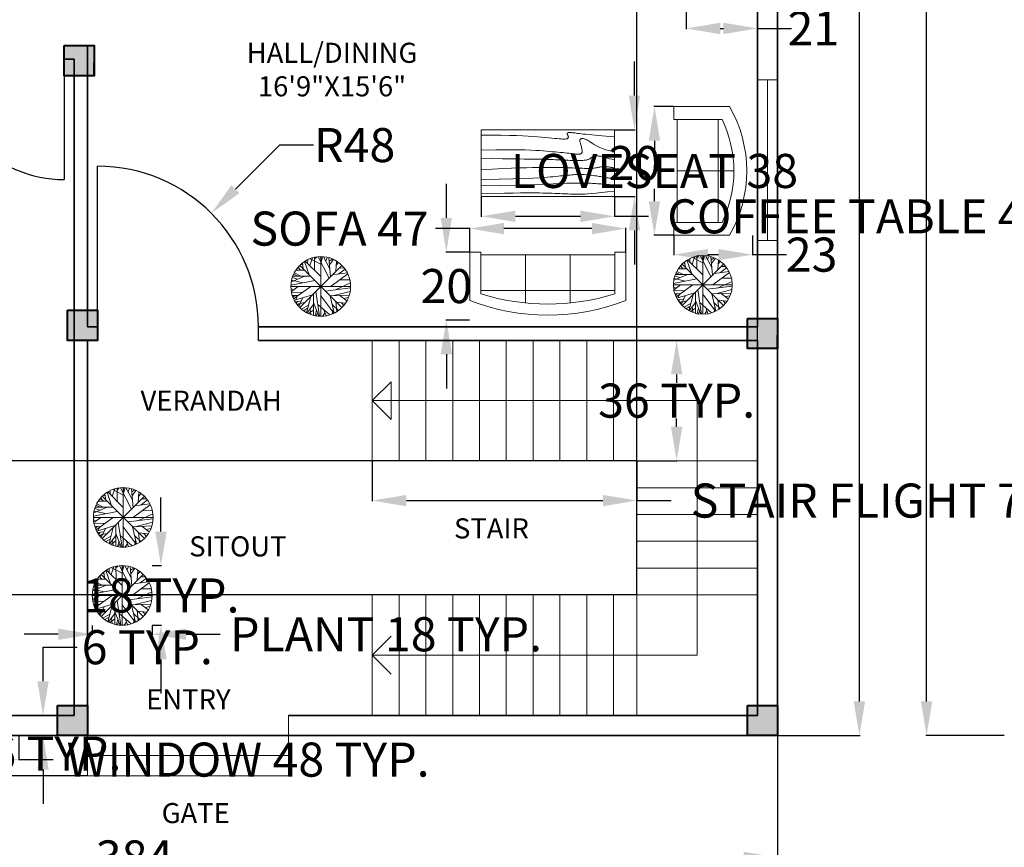
# Model space of a CAD drawing. Units: inches. Extents: x -107 to 647, y -210 to 500.
# Tile 4 of 7: x 183 to 477, y -31 to 216. Entities that reach past the tile are written whole.
import ezdxf

# ---------------------------------------------------------------- set-up
doc = ezdxf.new("R2010")
doc.units = ezdxf.units.IN
doc.header["$MEASUREMENT"] = 0
for name, color, linetype, lineweight in [('A-ANNO-DIMS', 2, 'Continuous', 18), ('A-ANNO-SYMB', 2, 'Continuous', 13), ('A-ANNO-TEXT', 7, 'Continuous', 18), ('A-AREA-IDEN', 7, 'Continuous', 18), ('A-COLS', 7, 'Continuous', 40), ('A-DOOR', 3, 'Continuous', 25), ('A-FLOR-STRS', 7, 'Continuous', 18), ('A-FURN', 8, 'Continuous', 18), ('A-GLAZ', 4, 'Continuous', 18), ('A-WALL', 7, 'Continuous', 35), ('L-PLNT', 3, 'Continuous', 13)]:
    doc.layers.add(name, color=color, linetype=linetype, lineweight=lineweight)
doc.styles.get("Standard").update_dxf_attribs({"font": 'arial.ttf'})
doc.dimstyles.get("Standard").update_dxf_attribs({"dimtxt": 10.18, "dimasz": 10.18, "dimexe": 0.18, "dimexo": 0.0625, "dimgap": 0.09, "dimtad": 0, "dimtih": 1, "dimtoh": 1, "dimdec": 0, "dimzin": 0, "dimdsep": 46, "dimlunit": 3, "dimtxsty": 'Standard', "dimcen": 0.09, "dimadec": 0, "dimazin": 0, "dimtfac": 1, "dimtdec": 0, "dimtofl": 0, "dimtmove": 0, "dimatfit": 3, "dimfxl": 1, "dimtolj": 1, "dimtzin": 0, "dimarcsym": 0})

# ---------------------------------------------------------------- blocks, each defined once
blk = doc.blocks.new('Sofa - Roundback 7 ft.')
for p, q in [((-12.00002, -32.4421), (-12.00003, -6.5971)), ((11.99997, -32.4421), (11.99998, -6.5971)), ((-36.000027, -34), (-36.000027, -11.4696)), ((-35.999844, -13.3819), (35.9998, -13.3819)), ((35.99998, -34), (35.99998, -11.4696)), ((-36.000027, -32.4421), (35.99998, -32.4421))]:
    blk.add_line(p, q)
for points in [[(-36.000027, -34), (-42.000027, -34), (-42.000027, -8)], [(41.99998, -8), (41.99998, -34), (35.99998, -34)]]:
    blk.add_lwpolyline(points)
for centre, radius, start, end in [((0, -114.25), 114.25, 68.43141, 111.5686), ((-0.00001, -127.1968), 121.1968, 72.72033, 107.2797)]:
    blk.add_arc(centre, radius, start, end)
blk = doc.blocks.new('Sofa - Roundback Loveseat 5 ft.')
for p, q in [((0, -32.44198), (0, -5.99998)), ((-24, -33.99998), (-24, -11.46958)), ((-23.9998, -13.38178), (23.99986, -13.38178)), ((24.00004, -33.99998), (24.00004, -11.46958)), ((-24, -32.44198), (24.00004, -32.44198))]:
    blk.add_line(p, q)
for points in [[(-24, -33.99998), (-30, -33.99998), (-30, -7.99998)], [(30.00004, -7.99998), (30.00004, -33.99998), (24.00004, -33.99998)]]:
    blk.add_lwpolyline(points)
for centre, radius, start, end in [((0, -60.24998), 60.24998, 60.13715, 119.8628), ((0, -61.38438), 55.38444, 64.32083, 115.6792)]:
    blk.add_arc(centre, radius, start, end)
blk = doc.blocks.new('Table - Rectangular Woodgrain 60 x 30 in.')
for p, q in [((0, 0), (0, -30)), ((60, 0), (0, 0)), ((60, -30), (60, 0)), ((0, -30), (60, -30))]:
    blk.add_line(p, q)
for points in [[(0, -2.4), (4.8155, -2.418), (9.0302, -2.4688), (12.709, -2.5477), (15.9167, -2.65), (18.7181, -2.7711), (21.1781, -2.9063), (23.3616, -3.0508), (25.3333, -3.2), (27.1477, -3.3495), (28.8172, -3.4958), (30.3437, -3.636), (31.7291, -3.7667), (32.9756, -3.8849), (34.0849, -3.9875), (35.059, -4.0714), (35.9, -4.1334), (36.6114, -4.1711), (37.2041, -4.1854), (37.6906, -4.1779), (38.0833, -4.15), (38.3948, -4.1034), (38.6375, -4.0396), (38.8239, -3.9602), (38.9666, -3.8667), (39.0764, -3.7608), (39.1573, -3.6448), (39.2116, -3.521), (39.2416, -3.3917), (39.2498, -3.2593), (39.2385, -3.1261), (39.21, -2.9944), (39.1666, -2.8667), (39.111, -2.7447), (39.0468, -2.6281), (38.978, -2.5163), (38.9083, -2.4083), (38.8418, -2.3035), (38.7823, -2.201), (38.7337, -2.1001), (38.7, -2), (38.6844, -1.9003), (38.6875, -1.8021), (38.7094, -1.707), (38.75, -1.6167), (38.8094, -1.5326), (38.8875, -1.4563), (38.9844, -1.3893), (39.1, -1.3333), (39.2351, -1.2896), (39.3937, -1.2583), (39.5804, -1.2396), (39.8, -1.2333), (40.057, -1.2396), (40.3562, -1.2583), (40.7023, -1.2896), (41.1, -1.3333), (41.5547, -1.3895), (42.0755, -1.4573), (42.6721, -1.5361), (43.3542, -1.625), (44.1316, -1.7233), (45.014, -1.8302), (46.0114, -1.9449), (47.1333, -2.0667), (48.3862, -2.1947), (49.7625, -2.3281), (51.2513, -2.4663), (52.8416, -2.6083), (54.5226, -2.7535), (56.2833, -2.9011), (58.1127, -3.0501), (60, -3.2)], [(0, -9.2), (6.5759, -9.0858), (11.9385, -9.0365), (16.2527, -9.0418), (19.6833, -9.0917), (22.3952, -9.1759), (24.5531, -9.2844), (26.322, -9.4069), (27.8666, -9.5333), (29.3241, -9.6553), (30.7203, -9.7719), (32.0532, -9.8837), (33.3208, -9.9917), (34.5213, -10.0965), (35.6526, -10.199), (36.7128, -10.2999), (37.7, -10.4), (38.6129, -10.4996), (39.4531, -10.5969), (40.223, -10.6895), (40.925, -10.775), (41.5613, -10.8512), (42.1344, -10.9156), (42.6465, -10.966), (43.1, -11), (43.4976, -11.0158), (43.8437, -11.0136), (44.143, -10.9942), (44.4, -10.9583), (44.6195, -10.9069), (44.8062, -10.8406), (44.9648, -10.7603), (45.1, -10.6667), (45.2155, -10.5598), (45.3114, -10.4365), (45.3871, -10.2929), (45.4416, -10.125), (45.4743, -9.929), (45.4844, -9.7011), (45.4709, -9.4371), (45.4333, -9.1333), (45.3716, -8.7883), (45.2896, -8.4104), (45.1919, -8.0107), (45.0833, -7.6), (44.9685, -7.1893), (44.8521, -6.7896), (44.7388, -6.4117), (44.6333, -6.0667), (44.54, -5.7628), (44.4614, -5.4979), (44.4001, -5.2675), (44.3583, -5.0667), (44.3384, -4.8909), (44.3427, -4.7354), (44.3736, -4.5956), (44.4333, -4.4667), (44.5236, -4.3453), (44.6427, -4.2333), (44.7884, -4.1339), (44.9583, -4.05), (45.1501, -3.9849), (45.3614, -3.9417), (45.59, -3.9234), (45.8333, -3.9333), (46.0915, -3.9749), (46.3734, -4.0531), (46.6906, -4.1736), (47.0542, -4.3417), (47.4756, -4.5629), (47.9661, -4.8427), (48.5372, -5.1866), (49.2, -5.6), (49.9676, -6.0844), (50.8594, -6.625), (51.8965, -7.2031), (53.1, -7.8), (54.491, -8.3969), (56.0906, -8.975), (57.9199, -9.5156), (60, -10)], [(0, -12.8), (5.1847, -12.9322), (9.6213, -13.0323), (13.3963, -13.1059), (16.5958, -13.1583), (19.3063, -13.1952), (21.614, -13.2219), (23.6054, -13.2439), (25.3666, -13.2667), (26.9728, -13.2947), (28.4531, -13.3281), (29.8256, -13.3663), (31.1083, -13.4083), (32.3191, -13.4535), (33.476, -13.501), (34.597, -13.5501), (35.7, -13.6), (36.7984, -13.6497), (37.8875, -13.6979), (38.9578, -13.743), (40, -13.7833), (41.0047, -13.8174), (41.9625, -13.8438), (42.864, -13.8607), (43.7, -13.8667), (44.4631, -13.8604), (45.1552, -13.8417), (45.7801, -13.8104), (46.3416, -13.7667), (46.8439, -13.7104), (47.2906, -13.6417), (47.6858, -13.5604), (48.0333, -13.4667), (48.3375, -13.3608), (48.6042, -13.2448), (48.8396, -13.121), (49.05, -12.9917), (49.2417, -12.8593), (49.4208, -12.7261), (49.5937, -12.5944), (49.7667, -12.4667), (49.9452, -12.3451), (50.1323, -12.2313), (50.3303, -12.1268), (50.5416, -12.0333), (50.7686, -11.9524), (51.0135, -11.8854), (51.2788, -11.8341), (51.5666, -11.8), (51.8785, -11.7843), (52.2116, -11.7865), (52.562, -11.8059), (52.926, -11.8417), (53.2998, -11.8931), (53.6795, -11.9594), (54.0614, -12.0397), (54.4416, -12.1333), (54.8223, -12.2401), (55.2293, -12.3625), (55.6942, -12.5037), (56.2489, -12.6667), (56.9251, -12.8547), (57.7545, -13.0708), (58.7689, -13.3182), (60, -13.6)], [(0, -18), (5.124, -17.7273), (9.6609, -17.5057), (13.6705, -17.3303), (17.2125, -17.1958), (20.3467, -17.0973), (23.1328, -17.0297), (25.6307, -16.9878), (27.9, -16.9667), (29.9928, -16.9617), (31.9302, -16.9703), (33.7254, -16.9907), (35.3917, -17.0208), (36.9423, -17.0588), (38.3906, -17.1026), (39.7499, -17.1503), (41.0333, -17.2), (42.2519, -17.2496), (43.4073, -17.2969), (44.4986, -17.3395), (45.525, -17.375), (46.4858, -17.4012), (47.3802, -17.4156), (48.2074, -17.416), (48.9667, -17.4), (49.6583, -17.3662), (50.2872, -17.3167), (50.8595, -17.2547), (51.3812, -17.1833), (51.8584, -17.1057), (52.2971, -17.025), (52.7034, -16.9443), (53.0833, -16.8667), (53.443, -16.7951), (53.789, -16.7313), (54.128, -16.6768), (54.4666, -16.6334), (54.8115, -16.6024), (55.1693, -16.5854), (55.5465, -16.5841), (55.95, -16.6), (56.3828, -16.6337), (56.8346, -16.6823), (57.2915, -16.7418), (57.7396, -16.8084), (58.165, -16.878), (58.5539, -16.9469), (58.8924, -17.0111), (59.1666, -17.0667), (59.3679, -17.1107), (59.5078, -17.1438), (59.6032, -17.1675), (59.6708, -17.1833), (59.7275, -17.193), (59.7901, -17.1979), (59.8753, -17.1998), (60, -17.2)], [(0, -22.4), (8.0098, -22.2501), (14.4094, -22.1011), (19.4168, -21.9535), (23.25, -21.8083), (26.1269, -21.6663), (28.2656, -21.5281), (29.884, -21.3947), (31.2, -21.2667), (32.3967, -21.1448), (33.5172, -21.0292), (34.5697, -20.9198), (35.5625, -20.8167), (36.5037, -20.7198), (37.4015, -20.6292), (38.2642, -20.5448), (39.1, -20.4667), (39.9164, -20.3951), (40.7187, -20.3313), (41.5117, -20.2768), (42.3, -20.2333), (43.0883, -20.2024), (43.8812, -20.1854), (44.6836, -20.1841), (45.5, -20.2), (46.3328, -20.234), (47.1747, -20.2844), (48.0163, -20.3488), (48.8479, -20.425), (49.66, -20.5106), (50.4429, -20.6031), (51.1872, -20.7004), (51.8833, -20.8), (52.5246, -20.8999), (53.1166, -20.9995), (53.6681, -21.0983), (54.1875, -21.1958), (54.6834, -21.2919), (55.1646, -21.3859), (55.6394, -21.4777), (56.1167, -21.5667), (56.6028, -21.6515), (57.0961, -21.7266), (57.5929, -21.7852), (58.0896, -21.8208), (58.5823, -21.8268), (59.0674, -21.7964), (59.5412, -21.723), (60, -21.6)], [(0, -25.2), (8.6355, -25.0504), (15.7026, -24.9031), (21.4049, -24.7606), (25.9458, -24.625), (29.529, -24.4988), (32.3578, -24.3844), (34.6359, -24.284), (36.5667, -24.2), (38.3213, -24.1341), (39.9417, -24.0854), (41.437, -24.0523), (42.8167, -24.0333), (44.0901, -24.0268), (45.2667, -24.0313), (46.3557, -24.0451), (47.3667, -24.0667), (48.309, -24.0947), (49.1928, -24.1287), (50.0284, -24.168), (50.826, -24.2125), (51.5959, -24.2617), (52.3483, -24.3151), (53.0935, -24.3725), (53.8417, -24.4334), (54.6009, -24.497), (55.3699, -24.561), (56.1454, -24.6226), (56.9239, -24.6792), (57.7021, -24.7279), (58.4764, -24.7662), (59.2435, -24.7911), (60, -24.8)], [(0, -28.8), (5.6867, -28.6681), (10.45, -28.5698), (14.407, -28.5012), (17.675, -28.4584), (20.3711, -28.4374), (22.6125, -28.4344), (24.5164, -28.4455), (26.2, -28.4667), (27.762, -28.4947), (29.2276, -28.5281), (30.6033, -28.5663), (31.8958, -28.6084), (33.1118, -28.6535), (34.2578, -28.7011), (35.3405, -28.7501), (36.3666, -28.8), (37.3443, -28.8497), (38.288, -28.8974), (39.2137, -28.9412), (40.1375, -28.9792), (41.0753, -29.0093), (42.0432, -29.0297), (43.0572, -29.0384), (44.1333, -29.0333), (45.2936, -29.0114), (46.5843, -28.9641), (48.0579, -28.8816), (49.7666, -28.7542), (51.7629, -28.5721), (54.0989, -28.3255), (56.8272, -28.0048), (60, -27.6)]]:
    blk.add_lwpolyline(points)
blk = doc.blocks.new('Tree - deciduous plan')
for p, q in [((-12.5388, 54.9406), (-7.9613, 59.4546)), ((-5.3205, 59.6806), (16.5105, 16.7963)), ((2.426, 54.9406), (-1.4472, 59.9056)), ((0, 59.9996), (0, -60)), ((0.4894, 48.6208), (3.6584, 59.6806)), ((18.2711, 35.5298), (5.419, 59.6806)), ((-43.8768, 36.4326), (-44.405, 40.2696)), ((42, 42), (-42, -42)), ((42, -42), (-42, 42)), ((-40.1797, 44.558), (-36.4825, 43.2038)), ((-37.0107, 47.0408), (-35.25, 35.5298)), ((-32.6092, 50.4264), (-23.2782, 23.5674)), ((-31.2008, 51.1035), (-0.2149, 20.1818)), ((-26.4472, 46.5894), (-26.2712, 53.8116)), ((-22.0458, 42.0753), (-16.5881, 57.6486)), ((-21.1656, 55.8436), (-0.0388, 45.0094)), ((-12.3627, 32.1443), (-12.5388, 58.7776)), ((9.8203, 51.5549), (12.8133, 58.5516)), ((19.6795, 19.5047), (16.3344, 57.6486)), ((17.0387, 51.1035), (23.2006, 55.1666)), ((17.7429, 43.6552), (25.4894, 54.2636)), ((31.6513, 50.8778), (30.2429, 30.5643)), ((31.1232, 42.5267), (35.8767, 48.1693)), ((-32.2571, 20.6333), (-59.1937, 9.348)), ((-56.0247, 20.859), (-20.8134, 20.859)), ((-54.7923, 24.4702), (-47.75, 21.0847)), ((-53.2078, 27.4044), (-40.1797, 20.859)), ((-49.8627, 32.8214), (-32.7853, 32.8214)), ((-45.8134, 38.2383), (-40.5318, 33.0471)), ((54.3626, 25.3731), (20.9119, 0.3198)), ((23.3767, 23.3417), (53.3063, 27.4044)), ((36.2288, 25.1474), (48.9049, 35.0784)), ((37.1091, 37.1098), (46.6161, 37.5612)), ((-59.7219, 2.8025), (-12.0106, 12.0565)), ((-58.6656, 12.7336), (-35.9543, 7.5424)), ((-57.081, 17.9248), (-47.0458, 14.7649)), ((-54.6162, -24.7335), (-20.2853, 0.0941)), ((29.3626, -6.6771), (59.4682, 7.091)), ((38.5175, 13.4107), (58.2359, 13.6364)), ((-60, 0), (60, 0)), ((-59.7219, -4.8714), (-54.2641, -6.6771)), ((-45.2853, -0.1316), (-59.0177, -10.0627)), ((-58.4895, -12.3197), (-36.4825, -11.6426)), ((-57.081, -18.4138), (-45.2853, -17.9624)), ((-52.6797, -18.188), (-55.4966, -22.0251)), ((-53.2078, -27.442), (-16.7641, -16.6081)), ((-47.2219, -19.3166), (-50.2148, -26.3135)), ((-14.8275, -15.0282), (-14.6515, -57.6865)), ((-10.074, -10.0627), (-2.5036, -59.7178)), ((-0.0388, -19.0909), (25.8415, -53.8495)), ((9.2922, -9.1598), (59.6443, -2.8401)), ((18.6232, -18.6394), (26.7218, -53.3981)), ((18.7992, -18.6394), (57.3556, -17.2853)), ((26.3697, -18.4138), (58.9401, -9.8369)), ((38.1654, -18.188), (52.426, -29.0219)), ((-38.9472, -29.0219), (-51.4472, -30.6018)), ((-46.5177, -30.1504), (-49.5106, -33.536)), ((-32.4331, -32.4075), (-48.1021, -35.5674)), ((-43.7008, -34.6645), (-46.6937, -37.373)), ((-35.9543, -22.4765), (-44.0529, -40.5329)), ((-24.6867, -37.8244), (-38.7712, -45.7241)), ((-19.9331, -20.2194), (-28.5599, -52.721)), ((-14.6515, -36.2445), (-27.6797, -52.9467)), ((-14.6515, -32.1818), (-3.912, -59.4922)), ((-6.2008, -36.2445), (17.919, -57.0094)), ((22.8485, -36.4702), (35.3485, -48.4326)), ((30.419, -30.1504), (32.3556, -50.0125)), ((31.4753, -31.279), (49.6091, -33.3103)), ((41.5105, -32.6332), (46.088, -38.0501)), ((45.9119, -24.0564), (55.595, -22.2508)), ((-26.2712, -43.9185), (-34.7219, -48.6583)), ((-14.6515, -47.3041), (-25.0388, -54.3009)), ((-21.5177, -45.4984), (-19.9331, -56.1065)), ((-8.4895, -47.5298), (-11.4825, -58.5893)), ((-6.3768, -52.721), (-9.3698, -58.815)), ((8.4119, -53.1724), (3.8344, -59.4922)), ((5.9471, -46.6269), (10.5246, -58.5893)), ((24.7852, -44.8213), (23.0246, -54.978))]:
    blk.add_line(p, q)
blk.add_circle((0, 0), 60)
blk = doc.blocks.new('DOOR-SWING-36IN')
for p, q in [((-36, 4), (-36, 0)), ((0, 4), (0, 0)), ((0, 0), (0, -36))]:
    blk.add_line(p, q)
blk.add_arc((0, 0), 36, 180, 270)
blk = doc.blocks.new('WINDOW-48IN')
for p, q in [((0, 6), (0, 0)), ((48, 6), (48, 0)), ((0, 3), (48, 3))]:
    blk.add_line(p, q)
blk = doc.blocks.new('STAIR-FLIGHT-36IN')
for p, q in [((0, 36), (0, 0)), ((8, 36), (8, 0)), ((16, 36), (16, 0)), ((24, 36), (24, 0)), ((32, 36), (32, 0)), ((40, 36), (40, 0)), ((48, 36), (48, 0)), ((56, 36), (56, 0)), ((64, 36), (64, 0)), ((72, 36), (72, 0)), ((79, 0), (0, 0))]:
    blk.add_line(p, q)
blk = doc.blocks.new('COLUMN-9X9IN')
blk.add_lwpolyline([(0, 9), (9, 9), (9, 0), (0, 0)], close=True)
blk.add_solid([(0, 9), (0, 0), (9, 9), (9, 0)])
blk = doc.blocks.new('COLUMN-9X9IN-CORNER-MARK')
for q in [(9, 4), (6, 0)]:
    blk.add_line((9, 0), q)
blk.add_lwpolyline([(0, 9), (9, 9), (9, 0), (0, 0)], close=True)
blk.add_solid([(0, 9), (0, 0), (9, 9), (9, 0)])
blk = doc.blocks.new('*D26')
at = {"layer": 'A-ANNO-DIMS', "color": 0, "lineweight": -2, "transparency": 16777216}
for p, q in [((134.58, 2.26), (134.58, -5.05)), ((182.58, 2.26), (182.58, -5.05)), ((144.76, -4.87), (172.4, -4.87)), ((182.58, -4.87), (192.76, -4.87))]:
    blk.add_line(p, q, dxfattribs=at)
at = {"layer": 'A-ANNO-DIMS', "color": 0, "transparency": 16777216}
for points in [[(144.76, -3.18), (144.76, -6.57), (134.58, -4.87)], [(172.4, -3.18), (172.4, -6.57), (182.58, -4.87)]]:
    blk.add_solid(points, dxfattribs=at)
at = {"layer": 'Defpoints', "color": 0, "transparency": 16777216}
for p in [(134.58, 2.33), (182.58, 2.33), (182.58, -4.87)]:
    blk.add_point(p, dxfattribs=at)
at = {"layer": 'A-ANNO-DIMS', "color": 0, "transparency": 16777216, "insert": (251.01, -4.87), "char_height": 10.18, "attachment_point": 5}
blk.add_mtext('\\A1;WINDOW 48 TYP.', dxfattribs=at)
blk = doc.blocks.new('*D27')
at = {"layer": 'A-ANNO-DIMS', "color": 0, "lineweight": -2, "transparency": 16777216}
for p, q in [((189.78, 18.51), (189.78, 28.69)), ((189.78, 28.69), (199.96, 28.69)), ((182.64, 8.33), (189.96, 8.33)), ((182.64, 2.33), (189.96, 2.33)), ((189.78, -7.85), (189.78, -18.03))]:
    blk.add_line(p, q, dxfattribs=at)
at = {"layer": 'A-ANNO-DIMS', "color": 0, "transparency": 16777216}
for points in [[(188.09, 18.51), (191.48, 18.51), (189.78, 8.33)], [(188.09, -7.85), (191.48, -7.85), (189.78, 2.33)]]:
    blk.add_solid(points, dxfattribs=at)
at = {"layer": 'Defpoints', "color": 0, "transparency": 16777216}
for p in [(182.58, 8.33), (189.78, 8.33), (182.58, 2.33)]:
    blk.add_point(p, dxfattribs=at)
at = {"layer": 'A-ANNO-DIMS', "color": 0, "transparency": 16777216, "insert": (220.9, 28.69), "char_height": 10.18, "attachment_point": 5}
blk.add_mtext('\\A1;6 TYP.', dxfattribs=at)
blk = doc.blocks.new('*D28')
at = {"layer": 'A-ANNO-DIMS', "color": 0, "lineweight": -2, "transparency": 16777216}
for p, q in [((54.58, 2.26), (54.58, -3.25)), ((90.58, 2.26), (90.58, -3.25)), ((64.76, -3.07), (80.4, -3.07)), ((90.58, -3.07), (100.76, -3.07))]:
    blk.add_line(p, q, dxfattribs=at)
at = {"layer": 'A-ANNO-DIMS', "color": 0, "transparency": 16777216}
for points in [[(64.76, -1.38), (64.76, -4.77), (54.58, -3.07)], [(80.4, -1.38), (80.4, -4.77), (90.58, -3.07)]]:
    blk.add_solid(points, dxfattribs=at)
at = {"layer": 'Defpoints', "color": 0, "transparency": 16777216}
for p in [(54.58, 2.33), (90.58, 2.33), (90.58, -3.07)]:
    blk.add_point(p, dxfattribs=at)
at = {"layer": 'A-ANNO-DIMS', "color": 0, "transparency": 16777216, "insert": (159.01, -3.07), "char_height": 10.18, "attachment_point": 5}
blk.add_mtext('\\A1;WINDOW 36 TYP.', dxfattribs=at)
blk = doc.blocks.new('*D48')
at = {"layer": 'A-ANNO-DIMS', "color": 0, "lineweight": -2, "transparency": 16777216}
for p, q in [((288.08, 84.26), (288.08, 72.3)), ((367.08, 84.26), (367.08, 72.3)), ((298.26, 72.48), (356.9, 72.48)), ((367.08, 72.48), (377.26, 72.48))]:
    blk.add_line(p, q, dxfattribs=at)
at = {"layer": 'A-ANNO-DIMS', "color": 0, "transparency": 16777216}
for points in [[(298.26, 74.17), (298.26, 70.78), (288.08, 72.48)], [(356.9, 74.17), (356.9, 70.78), (367.08, 72.48)]]:
    blk.add_solid(points, dxfattribs=at)
at = {"layer": 'Defpoints', "color": 0, "transparency": 16777216}
for p in [(288.08, 84.33), (367.08, 84.33), (367.08, 72.48)]:
    blk.add_point(p, dxfattribs=at)
at = {"layer": 'A-ANNO-DIMS', "color": 0, "transparency": 16777216, "insert": (452.28, 72.48), "char_height": 10.18, "attachment_point": 5}
blk.add_mtext('\\A1;STAIR FLIGHT 79 TYP.', dxfattribs=at)
blk = doc.blocks.new('*D49')
at = {"layer": 'A-ANNO-DIMS', "color": 0, "lineweight": -2, "transparency": 16777216}
for p, q in [((367.14, 120.33), (379.11, 120.33)), ((378.93, 110.15), (378.93, 107.62)), ((378.93, 94.51), (378.93, 97.03)), ((367.14, 84.33), (379.11, 84.33))]:
    blk.add_line(p, q, dxfattribs=at)
at = {"layer": 'A-ANNO-DIMS', "color": 0, "transparency": 16777216}
for points in [[(377.24, 110.15), (380.63, 110.15), (378.93, 120.33)], [(377.24, 94.51), (380.63, 94.51), (378.93, 84.33)]]:
    blk.add_solid(points, dxfattribs=at)
at = {"layer": 'Defpoints', "color": 0, "transparency": 16777216}
for p in [(367.08, 120.33), (378.93, 120.33), (367.08, 84.33)]:
    blk.add_point(p, dxfattribs=at)
at = {"layer": 'A-ANNO-DIMS', "color": 0, "transparency": 16777216, "insert": (378.93, 102.33), "char_height": 10.18, "attachment_point": 5}
blk.add_mtext('\\A1;36 TYP.', dxfattribs=at)
blk = doc.blocks.new('*D54')
at = {"layer": 'A-ANNO-DIMS', "color": 0, "lineweight": -2, "transparency": 16777216}
for p, q in [((317.17, 153.7), (306.99, 153.7)), ((317.17, 146.76), (317.17, 153.88)), ((353.62, 153.7), (327.35, 153.7)), ((363.8, 146.76), (363.8, 153.88))]:
    blk.add_line(p, q, dxfattribs=at)
at = {"layer": 'A-ANNO-DIMS', "color": 0, "transparency": 16777216}
for points in [[(327.35, 155.39), (327.35, 152), (317.17, 153.7)], [(353.62, 155.39), (353.62, 152), (363.8, 153.7)]]:
    blk.add_solid(points, dxfattribs=at)
at = {"layer": 'Defpoints', "color": 0, "transparency": 16777216}
for p in [(317.17, 153.7), (317.17, 146.7), (363.8, 146.7)]:
    blk.add_point(p, dxfattribs=at)
at = {"layer": 'A-ANNO-DIMS', "color": 0, "transparency": 16777216, "insert": (278.3, 153.7), "char_height": 10.18, "attachment_point": 5}
blk.add_mtext('\\A1;SOFA 47', dxfattribs=at)
blk = doc.blocks.new('*D55')
at = {"layer": 'A-ANNO-DIMS', "color": 0, "lineweight": -2, "transparency": 16777216}
for p, q in [((310.18, 156.88), (310.18, 167.06)), ((317.11, 146.7), (310, 146.7)), ((317.11, 126.35), (310, 126.35)), ((310.18, 116.17), (310.18, 105.99))]:
    blk.add_line(p, q, dxfattribs=at)
at = {"layer": 'A-ANNO-DIMS', "color": 0, "transparency": 16777216}
for points in [[(308.48, 156.88), (311.88, 156.88), (310.18, 146.7)], [(308.48, 116.17), (311.88, 116.17), (310.18, 126.35)]]:
    blk.add_solid(points, dxfattribs=at)
at = {"layer": 'Defpoints', "color": 0, "transparency": 16777216}
for p in [(317.17, 146.7), (310.18, 126.35), (317.17, 126.35)]:
    blk.add_point(p, dxfattribs=at)
at = {"layer": 'A-ANNO-DIMS', "color": 0, "transparency": 16777216, "insert": (310.18, 136.53), "char_height": 10.18, "attachment_point": 5}
blk.add_mtext('\\A1;20', dxfattribs=at)
blk = doc.blocks.new('*D56')
at = {"layer": 'A-ANNO-DIMS', "color": 0, "lineweight": -2, "transparency": 16777216}
for p, q in [((378.01, 190.13), (372.13, 190.13)), ((372.31, 179.95), (372.31, 176.27)), ((372.31, 161.87), (372.31, 165.55)), ((378.01, 151.69), (372.13, 151.69))]:
    blk.add_line(p, q, dxfattribs=at)
at = {"layer": 'A-ANNO-DIMS', "color": 0, "transparency": 16777216}
for points in [[(370.61, 179.95), (374.01, 179.95), (372.31, 190.13)], [(370.61, 161.87), (374.01, 161.87), (372.31, 151.69)]]:
    blk.add_solid(points, dxfattribs=at)
at = {"layer": 'Defpoints', "color": 0, "transparency": 16777216}
for p in [(378.07, 190.13), (372.31, 151.69), (378.07, 151.69)]:
    blk.add_point(p, dxfattribs=at)
at = {"layer": 'A-ANNO-DIMS', "color": 0, "transparency": 16777216, "insert": (372.31, 170.91), "char_height": 10.18, "attachment_point": 5}
blk.add_mtext('\\A1;LOVESEAT 38', dxfattribs=at)
blk = doc.blocks.new('*D57')
at = {"layer": 'A-ANNO-DIMS', "color": 0, "lineweight": -2, "transparency": 16777216}
for p, q in [((378.07, 151.62), (378.07, 145.74)), ((401.57, 151.62), (401.57, 145.74)), ((388.25, 145.92), (391.39, 145.92)), ((401.57, 145.92), (411.75, 145.92))]:
    blk.add_line(p, q, dxfattribs=at)
at = {"layer": 'A-ANNO-DIMS', "color": 0, "transparency": 16777216}
for points in [[(388.25, 147.62), (388.25, 144.22), (378.07, 145.92)], [(391.39, 147.62), (391.39, 144.22), (401.57, 145.92)]]:
    blk.add_solid(points, dxfattribs=at)
at = {"layer": 'Defpoints', "color": 0, "transparency": 16777216}
for p in [(378.07, 151.69), (401.57, 151.69), (401.57, 145.92)]:
    blk.add_point(p, dxfattribs=at)
at = {"layer": 'A-ANNO-DIMS', "color": 0, "transparency": 16777216, "insert": (419.22, 145.92), "char_height": 10.18, "attachment_point": 5}
blk.add_mtext('\\A1;23', dxfattribs=at)
blk = doc.blocks.new('*D59')
at = {"layer": 'A-ANNO-DIMS', "color": 0, "lineweight": -2, "transparency": 16777216}
for p, q in [((381.75, 222.41), (381.75, 213.29)), ((403.08, 222.41), (403.08, 213.29)), ((391.93, 213.47), (392.9, 213.47)), ((403.08, 213.47), (413.26, 213.47))]:
    blk.add_line(p, q, dxfattribs=at)
at = {"layer": 'A-ANNO-DIMS', "color": 0, "transparency": 16777216}
for points in [[(391.93, 215.16), (391.93, 211.77), (381.75, 213.47)], [(392.9, 215.16), (392.9, 211.77), (403.08, 213.47)]]:
    blk.add_solid(points, dxfattribs=at)
at = {"layer": 'Defpoints', "color": 0, "transparency": 16777216}
for p in [(381.75, 222.47), (403.08, 222.47), (403.08, 213.47)]:
    blk.add_point(p, dxfattribs=at)
at = {"layer": 'A-ANNO-DIMS', "color": 0, "transparency": 16777216, "insert": (419.75, 213.47), "char_height": 10.18, "attachment_point": 5}
blk.add_mtext('\\A1;21', dxfattribs=at)
blk = doc.blocks.new('*D60')
at = {"layer": 'A-ANNO-DIMS', "color": 0, "lineweight": -2, "transparency": 16777216}
for p, q in [((320.6, 163.26), (320.6, 157.18)), ((360.38, 163.26), (360.38, 157.18)), ((330.78, 157.36), (350.2, 157.36)), ((360.38, 157.36), (370.56, 157.36))]:
    blk.add_line(p, q, dxfattribs=at)
at = {"layer": 'A-ANNO-DIMS', "color": 0, "transparency": 16777216}
for points in [[(330.78, 159.06), (330.78, 155.66), (320.6, 157.36)], [(350.2, 159.06), (350.2, 155.66), (360.38, 157.36)]]:
    blk.add_solid(points, dxfattribs=at)
at = {"layer": 'Defpoints', "color": 0, "transparency": 16777216}
for p in [(320.6, 163.33), (360.38, 163.33), (360.38, 157.36)]:
    blk.add_point(p, dxfattribs=at)
at = {"layer": 'A-ANNO-DIMS', "color": 0, "transparency": 16777216, "insert": (433.18, 157.36), "char_height": 10.18, "attachment_point": 5}
blk.add_mtext('\\A1;COFFEE TABLE 40', dxfattribs=at)
blk = doc.blocks.new('*D61')
at = {"layer": 'A-ANNO-DIMS', "color": 0, "lineweight": -2, "transparency": 16777216}
for p, q in [((366.34, 193.4), (366.34, 203.58)), ((360.44, 183.22), (366.52, 183.22)), ((360.44, 163.33), (366.52, 163.33)), ((366.34, 153.15), (366.34, 142.97))]:
    blk.add_line(p, q, dxfattribs=at)
at = {"layer": 'A-ANNO-DIMS', "color": 0, "transparency": 16777216}
for points in [[(364.65, 193.4), (368.04, 193.4), (366.34, 183.22)], [(364.65, 153.15), (368.04, 153.15), (366.34, 163.33)]]:
    blk.add_solid(points, dxfattribs=at)
at = {"layer": 'Defpoints', "color": 0, "transparency": 16777216}
for p in [(360.38, 183.22), (366.34, 183.22), (360.38, 163.33)]:
    blk.add_point(p, dxfattribs=at)
at = {"layer": 'A-ANNO-DIMS', "color": 0, "transparency": 16777216, "insert": (366.34, 173.27), "char_height": 10.18, "attachment_point": 5}
blk.add_mtext('\\A1;20', dxfattribs=at)
blk = doc.blocks.new('*D68')
at = {"layer": 'A-ANNO-DIMS', "color": 0, "lineweight": -2, "transparency": 16777216}
for p, q in [((194.31, 32.56), (184.13, 32.56)), ((204.49, 35.17), (204.49, 32.38)), ((222.32, 35.17), (222.32, 32.38)), ((232.5, 32.56), (242.68, 32.56))]:
    blk.add_line(p, q, dxfattribs=at)
at = {"layer": 'A-ANNO-DIMS', "color": 0, "transparency": 16777216}
for points in [[(194.31, 34.26), (194.31, 30.87), (204.49, 32.56)], [(232.5, 34.26), (232.5, 30.87), (222.32, 32.56)]]:
    blk.add_solid(points, dxfattribs=at)
at = {"layer": 'Defpoints', "color": 0, "transparency": 16777216}
for p in [(204.49, 35.24), (222.32, 35.24), (222.32, 32.56)]:
    blk.add_point(p, dxfattribs=at)
at = {"layer": 'A-ANNO-DIMS', "color": 0, "transparency": 16777216, "insert": (292.18, 32.56), "char_height": 10.18, "attachment_point": 5}
blk.add_mtext('\\A1;PLANT 18 TYP.', dxfattribs=at)
blk = doc.blocks.new('*D69')
at = {"layer": 'A-ANNO-DIMS', "color": 0, "lineweight": -2, "transparency": 16777216}
for p, q in [((224.99, 63.24), (224.99, 73.42)), ((222.38, 53.06), (225.17, 53.06)), ((222.38, 35.24), (225.17, 35.24)), ((224.99, 25.06), (224.99, 14.88))]:
    blk.add_line(p, q, dxfattribs=at)
at = {"layer": 'A-ANNO-DIMS', "color": 0, "transparency": 16777216}
for points in [[(223.29, 63.24), (226.69, 63.24), (224.99, 53.06)], [(223.29, 25.06), (226.69, 25.06), (224.99, 35.24)]]:
    blk.add_solid(points, dxfattribs=at)
at = {"layer": 'Defpoints', "color": 0, "transparency": 16777216}
for p in [(222.32, 53.06), (224.99, 53.06), (222.32, 35.24)]:
    blk.add_point(p, dxfattribs=at)
at = {"layer": 'A-ANNO-DIMS', "color": 0, "transparency": 16777216, "insert": (224.99, 44.15), "char_height": 10.18, "attachment_point": 5}
blk.add_mtext('\\A1;18 TYP.', dxfattribs=at)
blk = doc.blocks.new('*D72')
at = {"layer": 'A-ANNO-DIMS', "color": 0, "lineweight": -2, "transparency": 16777216}
for p, q in [((25.08, 2.26), (25.08, -34.27)), ((409.08, 2.26), (409.08, -34.27)), ((35.26, -34.09), (205.77, -34.09)), ((398.9, -34.09), (228.39, -34.09))]:
    blk.add_line(p, q, dxfattribs=at)
at = {"layer": 'A-ANNO-DIMS', "color": 0, "transparency": 16777216}
for points in [[(35.26, -32.39), (35.26, -35.79), (25.08, -34.09)], [(398.9, -32.39), (398.9, -35.79), (409.08, -34.09)]]:
    blk.add_solid(points, dxfattribs=at)
at = {"layer": 'Defpoints', "color": 0, "transparency": 16777216}
for p in [(25.08, 2.33), (409.08, 2.33), (409.08, -34.09)]:
    blk.add_point(p, dxfattribs=at)
at = {"layer": 'A-ANNO-DIMS', "color": 0, "transparency": 16777216, "insert": (217.08, -34.09), "char_height": 10.18, "attachment_point": 5}
blk.add_mtext('\\A1;384', dxfattribs=at)
blk = doc.blocks.new('*D73')
at = {"layer": 'A-ANNO-DIMS', "color": 0, "lineweight": -2, "transparency": 16777216}
for p, q in [((409.14, 464.33), (433.68, 464.33)), ((433.5, 454.15), (433.5, 238.61)), ((433.5, 12.51), (433.5, 228.04)), ((409.14, 2.33), (433.68, 2.33))]:
    blk.add_line(p, q, dxfattribs=at)
at = {"layer": 'A-ANNO-DIMS', "color": 0, "transparency": 16777216}
for points in [[(431.8, 454.15), (435.19, 454.15), (433.5, 464.33)], [(431.8, 12.51), (435.19, 12.51), (433.5, 2.33)]]:
    blk.add_solid(points, dxfattribs=at)
at = {"layer": 'Defpoints', "color": 0, "transparency": 16777216}
for p in [(409.08, 464.33), (433.5, 464.33), (409.08, 2.33)]:
    blk.add_point(p, dxfattribs=at)
at = {"layer": 'A-ANNO-DIMS', "color": 0, "transparency": 16777216, "insert": (433.5, 233.33), "char_height": 10.18, "attachment_point": 5}
blk.add_mtext('\\A1;462', dxfattribs=at)
blk = doc.blocks.new('*D74')
at = {"layer": 'A-ANNO-DIMS', "color": 0, "lineweight": -2, "transparency": 16777216}
for p, q in [((0.67, 12.51), (0.67, 22.69)), ((203.02, 2.33), (0.49, 2.33)), ((203.02, -9.67), (0.49, -9.67)), ((0.67, -19.85), (0.67, -30.03))]:
    blk.add_line(p, q, dxfattribs=at)
at = {"layer": 'A-ANNO-DIMS', "color": 0, "transparency": 16777216}
for points in [[(-1.03, 12.51), (2.36, 12.51), (0.67, 2.33)], [(-1.03, -19.85), (2.36, -19.85), (0.67, -9.67)]]:
    blk.add_solid(points, dxfattribs=at)
at = {"layer": 'Defpoints', "color": 0, "transparency": 16777216}
for p in [(0.67, 2.33), (203.08, 2.33), (203.08, -9.67)]:
    blk.add_point(p, dxfattribs=at)
at = {"layer": 'A-ANNO-DIMS', "color": 0, "transparency": 16777216, "insert": (0.67, -3.67), "char_height": 10.18, "attachment_point": 5}
blk.add_mtext('\\A1;12', dxfattribs=at)
blk = doc.blocks.new('*D80')
at = {"layer": 'A-ANNO-DIMS', "color": 0, "lineweight": -2, "transparency": 16777216}
for p, q in [((367.02, 84.33), (0.49, 84.33)), ((0.67, 74.15), (0.67, 69.61)), ((0.67, 54.51), (0.67, 59.04)), ((367.02, 44.33), (0.49, 44.33))]:
    blk.add_line(p, q, dxfattribs=at)
at = {"layer": 'A-ANNO-DIMS', "color": 0, "transparency": 16777216}
for points in [[(-1.03, 74.15), (2.36, 74.15), (0.67, 84.33)], [(-1.03, 54.51), (2.36, 54.51), (0.67, 44.33)]]:
    blk.add_solid(points, dxfattribs=at)
at = {"layer": 'Defpoints', "color": 0, "transparency": 16777216}
for p in [(0.67, 84.33), (367.08, 84.33), (367.08, 44.33)]:
    blk.add_point(p, dxfattribs=at)
at = {"layer": 'A-ANNO-DIMS', "color": 0, "transparency": 16777216, "insert": (0.67, 64.33), "char_height": 10.18, "attachment_point": 5}
blk.add_mtext('\\A1;40', dxfattribs=at)
blk = doc.blocks.new('*D81')
at = {"layer": 'A-ANNO-DIMS', "color": 0, "lineweight": -2, "transparency": 16777216}
for p, q in [((367.08, 44.39), (367.08, 488.92)), ((377.26, 488.74), (377.71, 488.74)), ((392.9, 488.74), (392.46, 488.74)), ((403.08, 44.39), (403.08, 488.92))]:
    blk.add_line(p, q, dxfattribs=at)
at = {"layer": 'A-ANNO-DIMS', "color": 0, "transparency": 16777216}
for points in [[(377.26, 490.44), (377.26, 487.04), (367.08, 488.74)], [(392.9, 490.44), (392.9, 487.04), (403.08, 488.74)]]:
    blk.add_solid(points, dxfattribs=at)
at = {"layer": 'Defpoints', "color": 0, "transparency": 16777216}
for p in [(403.08, 488.74), (367.08, 44.33), (403.08, 44.33)]:
    blk.add_point(p, dxfattribs=at)
at = {"layer": 'A-ANNO-DIMS', "color": 0, "transparency": 16777216, "insert": (385.08, 488.74), "char_height": 10.18, "attachment_point": 5}
blk.add_mtext('\\A1;36', dxfattribs=at)
blk = doc.blocks.new('*D98')
at = {"layer": 'A-ANNO-DIMS', "color": 0, "lineweight": -2, "transparency": 16777216}
for p, q in [((476.69, 464.33), (453.37, 464.33)), ((453.55, 454.15), (453.55, 238.61)), ((453.55, 12.51), (453.55, 228.04)), ((476.69, 2.33), (453.37, 2.33))]:
    blk.add_line(p, q, dxfattribs=at)
at = {"layer": 'A-ANNO-DIMS', "color": 0, "transparency": 16777216}
for points in [[(451.85, 454.15), (455.25, 454.15), (453.55, 464.33)], [(451.85, 12.51), (455.25, 12.51), (453.55, 2.33)]]:
    blk.add_solid(points, dxfattribs=at)
at = {"layer": 'Defpoints', "color": 0, "transparency": 16777216}
for p in [(453.55, 464.33), (476.75, 464.33), (476.75, 2.33)]:
    blk.add_point(p, dxfattribs=at)
at = {"layer": 'A-ANNO-DIMS', "color": 0, "transparency": 16777216, "insert": (453.55, 233.33), "char_height": 10.18, "attachment_point": 5}
blk.add_mtext('\\A1;462', dxfattribs=at)
blk = doc.blocks.new('*D103')
at = {"layer": 'A-ANNO-DIMS', "color": 0, "lineweight": -2, "transparency": 16777216}
for p, q in [((260.39, 178.63), (247.22, 165.46)), ((270.57, 178.63), (260.39, 178.63)), ((205.99, 124.33), (206.17, 124.33)), ((206.08, 124.24), (206.08, 124.42))]:
    blk.add_line(p, q, dxfattribs=at)
at = {"layer": 'A-ANNO-DIMS', "color": 0, "transparency": 16777216}
blk.add_solid([(246.02, 166.66), (248.42, 164.26), (240.02, 158.27)], dxfattribs=at)
at = {"layer": 'Defpoints', "color": 0, "transparency": 16777216}
for p in [(240.02, 158.27), (206.08, 124.33)]:
    blk.add_point(p, dxfattribs=at)
at = {"layer": 'A-ANNO-DIMS', "color": 0, "transparency": 16777216, "insert": (282.83, 178.63), "char_height": 10.18, "attachment_point": 5}
blk.add_mtext('\\A1;R48', dxfattribs=at)

msp = doc.modelspace()

# ---------------------------------------------------------------- linework, layer by layer
at = {"layer": 'A-ANNO-SYMB'}
for p, q in [((288.082, 102.325), (293.739, 107.982)), ((293.739, 107.982), (293.739, 96.668)), ((367.082, 102.325), (288.082, 102.325)), ((288.082, 102.325), (293.739, 96.668)), ((367.082, 102.325), (385.082, 102.325)), ((385.082, 26.325), (385.082, 102.325)), ((288.082, 26.325), (293.739, 31.982)), ((288.082, 26.325), (367.082, 26.325)), ((288.082, 26.325), (293.739, 20.668)), ((367.082, 26.325), (385.082, 26.325))]:
    msp.add_line(p, q, dxfattribs=at)
msp.add_solid([(288.082, 102.325), (293.739, 107.982), (293.739, 96.668), (288.082, 102.325)], dxfattribs=at)
at = {"layer": 'A-DOOR'}
for p, q in [((206.082, 124.325), (206.082, 172.325)), ((206.082, 120.325), (206.082, 124.325)), ((254.082, 120.325), (254.082, 124.325))]:
    msp.add_line(p, q, dxfattribs=at)
msp.add_arc((206.082, 124.325), 48, 0, 90, dxfattribs=at)
at = {"layer": 'A-FLOR-STRS'}
for p, q in [((367.082, 8.325), (367.082, 120.325)), ((367.082, 84.325), (403.082, 84.325)), ((367.082, 76.325), (403.082, 76.325)), ((367.082, 68.325), (403.082, 68.325)), ((367.082, 60.325), (403.082, 60.325)), ((367.082, 52.325), (403.082, 52.325)), ((367.082, 44.325), (403.082, 44.325)), ((203.082, 8.325), (203.082, -9.675)), ((263.082, 8.325), (263.082, -9.675))]:
    msp.add_line(p, q, dxfattribs=at)
for points in [[(203.082, -3.675), (263.082, -3.675)], [(203.082, -9.675), (263.082, -9.675)]]:
    msp.add_lwpolyline(points, dxfattribs=at)
at = {"layer": 'A-WALL'}
for p, q in [((403.082, 124.325), (403.082, 310.325)), ((203.082, 208.325), (196.082, 208.325)), ((203.082, 208.325), (203.082, 124.325)), ((199.082, 204.325), (196.082, 204.325)), ((199.082, 204.325), (199.082, 8.325)), ((206.082, 124.325), (203.082, 124.325)), ((403.082, 124.325), (254.082, 124.325)), ((203.082, 120.325), (203.082, 8.325)), ((206.082, 120.325), (203.082, 120.325)), ((403.082, 120.325), (254.082, 120.325)), ((403.082, 8.325), (403.082, 120.325)), ((118.082, 8.325), (199.082, 8.325)), ((263.082, 8.325), (403.082, 8.325))]:
    msp.add_line(p, q, dxfattribs=at)
msp.add_lwpolyline([(25.082, 2.325), (409.082, 2.325), (409.082, 464.325), (25.082, 464.325)], close=True, dxfattribs=at)

# ---------------------------------------------------------------- block references
at = {"layer": 'A-COLS'}
for name, p in [('COLUMN-9X9IN-CORNER-MARK', (196.082, 199.325)), ('COLUMN-9X9IN', (197.082, 120.325)), ('COLUMN-9X9IN-CORNER-MARK', (400.062, 117.898)), ('COLUMN-9X9IN', (194.082, 2.325)), ('COLUMN-9X9IN', (400.082, 2.325))]:
    msp.add_blockref(name, p, dxfattribs=at)
at = {"layer": 'A-DOOR'}
msp.add_blockref('DOOR-SWING-36IN', (196.082, 204.325), dxfattribs=at)
at = {"layer": 'A-FLOR-STRS'}
msp.add_blockref('STAIR-FLIGHT-36IN', (288.082, 84.325), dxfattribs=at)
at = {"layer": 'A-FLOR-STRS', "extrusion": (0, 0, -1), "zscale": -1, "rotation": 180}
msp.add_blockref('STAIR-FLIGHT-36IN', (-288.082, 44.325), dxfattribs=at)
at = {"layer": 'A-FURN'}
for name, p, xscale, yscale, zscale, rotation in [('Sofa - Roundback Loveseat 5 ft.', (399.858, 170.908), 0.6406987507126951, 0.6406987507126951, 0.6406987507126951, 269.9999754620093), ('Sofa - Roundback 7 ft.', (340.486, 127.829), 0.5550709472726072, 0.5550709472726072, 0.5550709472726072, 180)]:
    msp.add_blockref(name, p, dxfattribs=dict(at, xscale=xscale, yscale=yscale, zscale=zscale, rotation=rotation))
at = {"layer": 'A-FURN', "xscale": 0.6629571285703343, "yscale": 0.6629571285703343, "zscale": 0.6629571285703343}
msp.add_blockref('Table - Rectangular Woodgrain 60 x 30 in.', (320.599, 183.216), dxfattribs=at)
at = {"layer": 'A-GLAZ', "rotation": 269.9999999999998}
msp.add_blockref('WINDOW-48IN', (403.082, 198.148), dxfattribs=at)
at = {"layer": 'L-PLNT'}
for p, xscale, yscale, zscale in [((272.706, 136.412), 0.1485421662236593, 0.1485421662236593, 0.1485421662236593), ((386.75, 136.907), 0.146568951872548, 0.146568951872548, 0.146568951872548), ((213.728, 67.457), 0.1485421662236593, 0.1485421662236593, 0.1485421662236593), ((213.404, 44.149), 0.1485421662236593, 0.1485421662236593, 0.1485421662236593)]:
    msp.add_blockref('Tree - deciduous plan', p, dxfattribs=dict(at, xscale=xscale, yscale=yscale, zscale=zscale))

# ---------------------------------------------------------------- texts
at = {"layer": 'A-ANNO-TEXT', "char_height": 6, "attachment_point": 1}
for s, width, insert in [('\\pxqc;ENTRY', 29.58294, (218.384, 16.12)), ('\\pxqc;GATE', 25.39009, (222.67, -17.84))]:
    msp.add_mtext_dynamic_manual_height_columns(s, width=width, gutter_width=1, heights=[0], dxfattribs=dict(at, insert=insert))
at = {"layer": 'A-AREA-IDEN', "char_height": 6, "attachment_point": 1}
for s, width, insert in [('\\pxqc;HALL/DINING\\P16\'9"X15\'6"', 53.23254, (249.441, 209.194)), ('VERANDAH', 45.88849, (218.893, 105.295)), ('\\pxqc;STAIR', 25.39931, (310.953, 67.175)), ('\\pxqc;SITOUT', 33.27352, (231.311, 61.807))]:
    msp.add_mtext_dynamic_manual_height_columns(s, width=width, gutter_width=1, heights=[0], dxfattribs=dict(at, insert=insert))

# ---------------------------------------------------------------- dimensions: what is measured, and where the dimension line sits
at = {"layer": 'A-ANNO-DIMS'}
for base, p1, p2, picture, middle in [((403.082, 488.742), (367.082, 44.325), (403.082, 44.325), '*D81', (385.082, 488.742)), ((403.082, 213.468), (381.748, 222.468), (403.082, 222.468), '*D59', (419.747, 213.468)), ((409.082, -34.091), (25.082, 2.325), (409.082, 2.325), '*D72', (217.082, -34.091))]:
    dim = msp.add_linear_dim(base=base, p1=p1, p2=p2, dimstyle='Standard', override={"dimdec": 0, "dimlfac": 1, "dimrnd": 0, "dimzin": 0, "dimdsep": 46, "dimlunit": 2}, dxfattribs=at)
    dim.commit()
    dim.dimension.update_dxf_attribs({"geometry": picture, "text_midpoint": middle})
for base, p1, p2, angle, picture, middle in [((433.498, 464.325), (409.082, 2.325), (409.082, 464.325), 90, '*D73', (433.498, 233.325)), ((453.549, 464.325), (476.749, 2.325), (476.749, 464.325), 90, '*D98', (453.549, 233.325)), ((366.343, 183.216), (360.376, 163.327), (360.376, 183.216), 90, '*D61', (366.343, 173.271)), ((310.179, 126.349), (317.173, 146.702), (317.173, 126.349), 270, '*D55', (310.179, 136.525)), ((401.567, 145.921), (378.075, 151.687), (401.567, 151.687), 359.99998, '*D57', (419.215, 145.921)), ((0.665, 84.325), (367.082, 44.325), (367.082, 84.325), 90, '*D80', (0.665, 64.325)), ((0.665, 2.325), (203.082, -9.675), (203.082, 2.325), 90, '*D74', (0.665, -3.675))]:
    dim = msp.add_linear_dim(base=base, p1=p1, p2=p2, angle=angle, dimstyle='Standard', override={"dimdec": 0, "dimlfac": 1, "dimrnd": 0, "dimzin": 0, "dimdsep": 46, "dimlunit": 2}, dxfattribs=at)
    dim.commit()
    dim.dimension.update_dxf_attribs({"geometry": picture, "text_midpoint": middle})
for base, p1, p2, angle, text, picture, middle in [((372.308, 151.687), (378.075, 190.129), (378.075, 151.687), 269.99998, 'LOVESEAT <>', '*D56', (372.308, 170.908)), ((317.173, 153.696), (363.799, 146.702), (317.173, 146.702), 180, 'SOFA <>', '*D54', (278.3, 153.696)), ((378.932, 120.325), (367.082, 84.325), (367.082, 120.325), 90, '<> TYP.', '*D49', (378.932, 102.325)), ((224.99, 53.061), (222.316, 35.236), (222.316, 53.061), 90, '<> TYP.', '*D69', (224.99, 44.149)), ((189.782, 8.325), (182.582, 2.325), (182.582, 8.325), 90, '<> TYP.', '*D27', (220.901, 28.685))]:
    dim = msp.add_linear_dim(base=base, p1=p1, p2=p2, angle=angle, text=text, dimstyle='Standard', override={"dimdec": 0, "dimlfac": 1, "dimrnd": 0, "dimzin": 0, "dimdsep": 46, "dimlunit": 2}, dxfattribs=at)
    dim.commit()
    dim.dimension.update_dxf_attribs({"geometry": picture, "text_midpoint": middle})
dim = msp.add_radius_dim(center=(206.082, 124.325), mpoint=(240.023, 158.266), dimstyle='Standard', override={"dimdec": 0, "dimlfac": 1, "dimrnd": 0, "dimzin": 0, "dimdsep": 46, "dimlunit": 2}, dxfattribs=at)
dim.commit()
dim.dimension.update_dxf_attribs({"geometry": '*D103', "text_midpoint": (282.831, 178.631), "dimtype": 164})
for base, p1, p2, text, picture, middle in [((360.376, 157.36), (320.599, 163.327), (360.376, 163.327), 'COFFEE TABLE <>', '*D60', (433.177, 157.36)), ((367.082, 72.475), (288.082, 84.325), (367.082, 84.325), 'STAIR FLIGHT <> TYP.', '*D48', (452.278, 72.475)), ((222.316, 32.563), (204.491, 35.236), (222.316, 35.236), 'PLANT <> TYP.', '*D68', (292.184, 32.563)), ((90.582, -3.075), (54.582, 2.325), (90.582, 2.325), 'WINDOW <> TYP.', '*D28', (159.012, -3.075)), ((182.582, -4.875), (134.582, 2.325), (182.582, 2.325), 'WINDOW <> TYP.', '*D26', (251.012, -4.875))]:
    dim = msp.add_linear_dim(base=base, p1=p1, p2=p2, text=text, dimstyle='Standard', override={"dimdec": 0, "dimlfac": 1, "dimrnd": 0, "dimzin": 0, "dimdsep": 46, "dimlunit": 2}, dxfattribs=at)
    dim.commit()
    dim.dimension.update_dxf_attribs({"geometry": picture, "text_midpoint": middle})

doc.saveas('drawing.dxf')
